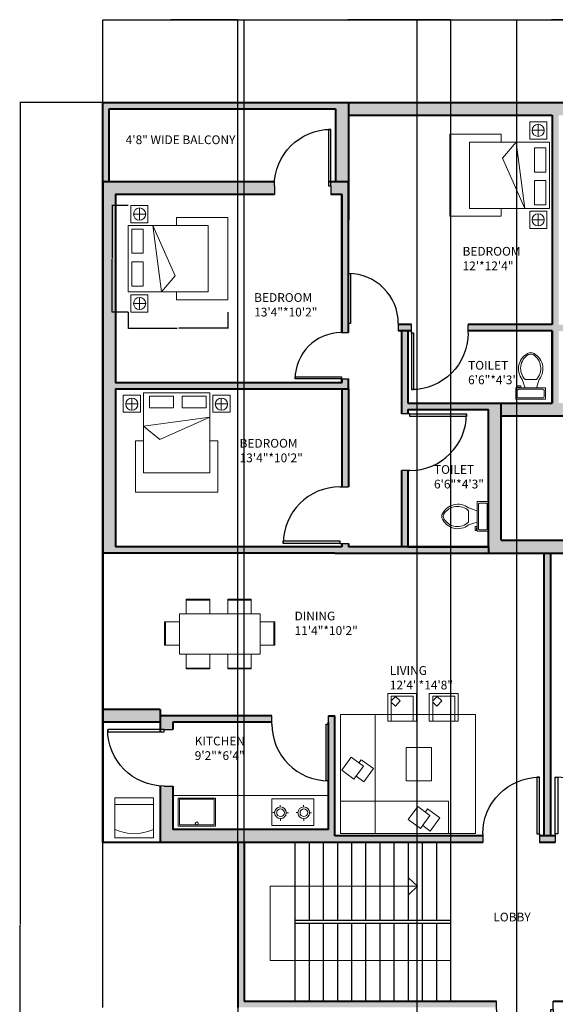
# Model space of a CAD drawing. Units: inches. Extents: x 1642 to 2399, y 1011 to 2291.
# Tile 4 of 7: x 1642 to 2020, y 1595 to 2291. Entities that reach past the tile are written whole.
import ezdxf

# ---------------------------------------------------------------- set-up
doc = ezdxf.new("R2010")
doc.units = ezdxf.units.IN
for name, color, linetype, lineweight in [('A-ANNO-DIMS', 2, 'Continuous', 18), ('A-ANNO-SYMB', 2, 'Continuous', 18), ('A-AREA-IDEN', 7, 'Continuous', 20), ('A-DOOR', 4, 'Continuous', 25), ('A-EQPM', 8, 'Continuous', 18), ('A-FLOR-CASE', 30, 'Continuous', 18), ('A-FLOR-FIXT', 9, 'Continuous', 18), ('A-FLOR-STRS', 7, 'Continuous', 25), ('A-FURN', 8, 'Continuous', 18), ('A-WALL-PATT', 40, 'Continuous', 13), ('BED', 200, 'Continuous', 18), ('WALL', 40, 'Continuous', 40)]:
    doc.layers.add(name, color=color, linetype=linetype, lineweight=lineweight)
doc.styles.get("Standard").update_dxf_attribs({"font": 'arial.ttf'})
doc.dimstyles.get("Standard").update_dxf_attribs({"dimtxt": 0.18, "dimasz": 0.18, "dimexe": 0.18, "dimexo": 0.0625, "dimgap": 0.09, "dimtad": 0, "dimtih": 1, "dimtoh": 1, "dimdec": 4, "dimzin": 0, "dimdsep": 46, "dimtxsty": 'Standard', "dimcen": 0.09, "dimadec": 0, "dimazin": 0, "dimtfac": 1, "dimtdec": 4, "dimtofl": 0, "dimtmove": 0, "dimatfit": 3, "dimfxl": 1, "dimtolj": 1, "dimtzin": 0, "dimarcsym": 0})

# ---------------------------------------------------------------- blocks, each defined once
blk = doc.blocks.new('*U2')
for p, q in [((0, 0), (0, -6)), ((40, 0), (40, -6))]:
    blk.add_line(p, q)
blk.add_lwpolyline([(0, 0), (0, 40), (1.75, 40), (1.75, 0)], close=True)
blk.add_arc((0, 0), 40, 0, 90)
blk = doc.blocks.new('*U4')
for p, q in [((9.5, -6), (9.5, -2)), ((-10, -8.5), (-8, -8.5)), ((-10, -9.5), (-10, -8.5)), ((-7, -9.5), (-10, -9.5)), ((-8, -8.5), (-8, -8)), ((-7, -8), (-7, -9.5)), ((-4, -8), (-6, -14)), ((4, -8), (6, -14)), ((4, -14), (-4, -14))]:
    blk.add_line(p, q)
blk.add_lwpolyline([(10.5, -8), (10.5, 0), (-10.5, 0), (-10.5, -8)], close=True)
for points in [[(-9.5, -2), (-9.5, -6)], [(8.5, -1), (-8.5, -1)], [(-8.5, -7), (8.5, -7)]]:
    blk.add_lwpolyline(points)
for centre, radius, start, end in [((-8.62, -1.88), 0.884, 81.8699, 188.1301), ((-8.62, -6.12), 0.884, 171.8699, 278.1301), ((8.62, -1.88), 0.884, 351.8699, 98.1301), ((8.62, -6.12), 0.884, 261.8699, 8.1301), ((3.52, -21.58), 12.17, 141.46911, 247.97143), ((4.2, -21.82), 11.33, 136.36773, 238.94682), ((-3.52, -21.58), 12.17, 292.02843, 38.53071), ((-4.2, -21.82), 11.33, 301.05301, 43.63209), ((0, -27.88), 4, 245.73182, 294.26817), ((0, -29), 4, 254.86053, 285.13947)]:
    blk.add_arc(centre, radius, start, end)
blk = doc.blocks.new('BED-DOUBLE-WITH-NIGHTSTANDS')
for p, q in [((8.62, 34.13), (8.62, 70.38)), ((8.62, 70.38), (66.79, 70.38)), ((66.79, 70.38), (66.79, 34.13)), ((14.22, 34.13), (8.62, 34.13)), ((14.22, 17.36), (49.69, 33.17)), ((49.69, 33.17), (61.11, 23.59)), ((66.79, 34.13), (61.11, 34.13)), ((61.11, 23.59), (14.22, 17.36)), ((1.82, 7.94), (10.42, 7.94)), ((6.17, 3.76), (6.17, 12.35)), ((65.06, 7.94), (73.65, 7.94)), ((69.41, 3.76), (69.41, 12.35))]:
    blk.add_line(p, q)
for points in [[(14.22, 0), (61.11, 0), (61.11, 56.52), (14.22, 56.52)], [(12.24, 1.79), (0, 1.79), (0, 13.82), (12.24, 13.82)], [(16.77, 2.51), (33.87, 2.51), (33.87, 10.66), (16.77, 10.66)], [(39.94, 2.51), (57.04, 2.51), (57.04, 10.66), (39.94, 10.66)], [(75.48, 1.79), (63.24, 1.79), (63.24, 13.82), (75.48, 13.82)]]:
    blk.add_lwpolyline(points, close=True)
for centre in [(6.12, 8.05), (69.36, 8.05)]:
    blk.add_circle(centre, 4.3)
blk = doc.blocks.new('TABLE-DINING-SIX-SEAT')
for p, q in [((15.31, 48.55), (31.81, 48.55)), ((44.68, 48.55), (61.18, 48.55)), ((0.59, 16.67), (0.59, 33.17)), ((77.22, 16.83), (77.22, 33.33)), ((15.31, 0.59), (31.81, 0.59)), ((44.68, 0.59), (61.18, 0.59))]:
    blk.add_line(p, q)
for points in [[(15.31, 38.77), (31.81, 38.77), (31.81, 49.15), (15.31, 49.15)], [(44.68, 38.77), (61.18, 38.77), (61.18, 49.15), (44.68, 49.15)], [(10.38, 38.77), (67.43, 38.77), (67.43, 10.38), (10.38, 10.38)], [(10.38, 16.67), (10.38, 33.17), (0, 33.17), (0, 16.67)], [(67.43, 16.83), (67.43, 33.33), (77.81, 33.33), (77.81, 16.83)], [(15.31, 10.38), (31.81, 10.38), (31.81, 0), (15.31, 0)], [(44.68, 10.38), (61.18, 10.38), (61.18, 0), (44.68, 0)]]:
    blk.add_lwpolyline(points, close=True)
blk = doc.blocks.new('SEATING-CORNER')
for points in [[(0, 84.13), (76.26, 84.13), (76.26, 61.34), (0, 61.34)], [(0, 0), (24.56, 0), (24.56, 84.13), (0, 84.13)], [(56.51, 80.66), (63.26, 71.39), (54.61, 65.09), (47.86, 74.37)], [(9.57, 45.8), (16.32, 36.53), (7.67, 30.23), (0.92, 39.51)]]:
    blk.add_lwpolyline(points, close=True)
for points in [[(58.1, 78.48), (63.51, 82.42), (70.26, 73.15), (61.61, 66.85), (60.02, 69.03)], [(11.16, 43.62), (16.57, 47.56), (23.32, 38.28), (14.67, 31.99), (13.08, 34.17)]]:
    blk.add_lwpolyline(points)
blk = doc.blocks.new('CHAIR-LOUNGE')
for p, q in [((2.54, 19.51), (0, 19.51)), ((0, 19.51), (0, 0)), ((18.08, 19.51), (20.31, 19.51)), ((20.31, 19.32), (20.31, 19.51)), ((20.31, 0), (20.31, 19.32)), ((0, 0), (20.31, 0))]:
    blk.add_line(p, q)
blk.add_lwpolyline([(2.54, 19.51), (18.08, 19.51), (18.08, 1.93), (2.54, 1.93)], close=True)
blk.add_lwpolyline([(2.54, 6.05), (5.4, 8.82), (8.88, 5.23), (5.55, 2), (2.54, 5.1)])
blk = doc.blocks.new('COOKTOP-TWO-BURNER')
for p, q in [((6.17, 13.89), (6.17, 15.59)), ((22.64, 13.89), (22.64, 15.59)), ((2, 9.67), (0.69, 9.67)), ((10.24, 9.72), (11.69, 9.72)), ((18.47, 9.67), (17.17, 9.67)), ((26.71, 9.72), (28.17, 9.72)), ((6.02, 5.65), (6.02, 4.35)), ((22.49, 5.65), (22.49, 4.35))]:
    blk.add_line(p, q)
blk.add_lwpolyline([(0, 18.89), (29.66, 18.89), (29.66, 0), (0, 0)], close=True)
for centre, radius in [((6.12, 9.77), 4.12), ((6.17, 9.77), 2.71), ((22.59, 9.77), 4.12), ((22.64, 9.77), 2.71)]:
    blk.add_circle(centre, radius)
blk = doc.blocks.new('SINK-KITCHEN-SINGLE')
for points in [[(0, 19.82), (26.24, 19.82), (26.24, 0), (0, 0)], [(0.83, 18.98), (25.41, 18.98), (25.41, 0.83), (0.83, 0.83)]]:
    blk.add_lwpolyline(points, close=True)
blk.add_circle((13.12, 17.93), 1.05)
blk = doc.blocks.new('UTILITY-APPLIANCE')
blk.add_line((0, 4.7), (27.35, 4.7))
blk.add_lwpolyline([(0, 28.26), (27.35, 28.26), (27.35, 0), (0, 0)], close=True)
blk.add_arc((13.68, -6.28), 31.65, 64.3994, 115.6006)
blk = doc.blocks.new('TABLE-COFFEE')
blk.add_lwpolyline([(0, 23.65), (17.89, 23.65), (17.89, 0), (0, 0)], close=True)
blk = doc.blocks.new('*D14')
at = {"layer": 'A-ANNO-DIMS', "color": 0, "lineweight": -2, "transparency": 16777216}
for p, q in [((1718.62, 2159.7), (1707.18, 2159.7)), ((1707.36, 2159.52), (1707.36, 2122.14)), ((1707.36, 2084.4), (1707.36, 2121.78)), ((1718.62, 2084.22), (1707.18, 2084.22))]:
    blk.add_line(p, q, dxfattribs=at)
at = {"layer": 'A-ANNO-DIMS', "color": 0, "transparency": 16777216}
for points in [[(1707.33, 2159.52), (1707.39, 2159.52), (1707.36, 2159.7)], [(1707.33, 2084.4), (1707.39, 2084.4), (1707.36, 2084.22)]]:
    blk.add_solid(points, dxfattribs=at)
at = {"layer": 'Defpoints', "color": 0, "transparency": 16777216}
for p in [(1718.68, 2159.7), (1707.36, 2084.22), (1718.68, 2084.22)]:
    blk.add_point(p, dxfattribs=at)
at = {"layer": 'A-ANNO-DIMS', "color": 0, "transparency": 16777216, "insert": (1707.36, 2121.96), "char_height": 0.18, "attachment_point": 5}
blk.add_mtext('\\A1;BED 75 TYP.', dxfattribs=at)
blk = doc.blocks.new('*D15')
at = {"layer": 'A-ANNO-DIMS', "color": 0, "lineweight": -2, "transparency": 16777216}
for p, q in [((1718.68, 2084.16), (1718.68, 2072.72)), ((1789.06, 2084.16), (1789.06, 2072.72)), ((1718.86, 2072.9), (1753.35, 2072.9)), ((1788.88, 2072.9), (1754.4, 2072.9))]:
    blk.add_line(p, q, dxfattribs=at)
at = {"layer": 'A-ANNO-DIMS', "color": 0, "transparency": 16777216}
for points in [[(1718.86, 2072.93), (1718.86, 2072.87), (1718.68, 2072.9)], [(1788.88, 2072.93), (1788.88, 2072.87), (1789.06, 2072.9)]]:
    blk.add_solid(points, dxfattribs=at)
at = {"layer": 'Defpoints', "color": 0, "transparency": 16777216}
for p in [(1718.68, 2084.22), (1789.06, 2084.22), (1789.06, 2072.9)]:
    blk.add_point(p, dxfattribs=at)
at = {"layer": 'A-ANNO-DIMS', "color": 0, "transparency": 16777216, "insert": (1753.87, 2072.9), "char_height": 0.18, "attachment_point": 5}
blk.add_mtext('\\A1;70 TYP.', dxfattribs=at)
blk = doc.blocks.new('*D32')
at = {"layer": 'A-ANNO-DIMS', "color": 0, "lineweight": -2, "transparency": 16777216}
for p, q in [((1700.71, 2232.52), (1700.71, 2290.98)), ((1700.89, 2290.8), (2020.07, 2290.8)), ((2340.03, 2290.8), (2020.86, 2290.8)), ((2340.21, 2232.52), (2340.21, 2290.98))]:
    blk.add_line(p, q, dxfattribs=at)
at = {"layer": 'A-ANNO-DIMS', "color": 0, "transparency": 16777216}
for points in [[(1700.89, 2290.83), (1700.89, 2290.77), (1700.71, 2290.8)], [(2340.03, 2290.83), (2340.03, 2290.77), (2340.21, 2290.8)]]:
    blk.add_solid(points, dxfattribs=at)
at = {"layer": 'Defpoints', "color": 0, "transparency": 16777216}
for p in [(2340.21, 2290.8), (1700.71, 2232.46), (2340.21, 2232.46)]:
    blk.add_point(p, dxfattribs=at)
at = {"layer": 'A-ANNO-DIMS', "color": 0, "transparency": 16777216, "insert": (2020.46, 2290.8), "char_height": 0.18, "attachment_point": 5}
blk.add_mtext('\\A1;639.5', dxfattribs=at)
blk = doc.blocks.new('*D33')
at = {"layer": 'A-ANNO-DIMS', "color": 0, "lineweight": -2, "transparency": 16777216}
for p, q in [((1700.65, 2232.46), (1642.19, 2232.46)), ((1642.37, 2232.28), (1642.37, 1651.26)), ((1642.37, 1069.89), (1642.37, 1650.9)), ((1700.65, 1069.71), (1642.19, 1069.71))]:
    blk.add_line(p, q, dxfattribs=at)
at = {"layer": 'A-ANNO-DIMS', "color": 0, "transparency": 16777216}
for points in [[(1642.34, 2232.28), (1642.4, 2232.28), (1642.37, 2232.46)], [(1642.34, 1069.89), (1642.4, 1069.89), (1642.37, 1069.71)]]:
    blk.add_solid(points, dxfattribs=at)
at = {"layer": 'Defpoints', "color": 0, "transparency": 16777216}
for p in [(1642.37, 2232.46), (1700.71, 2232.46), (1700.71, 1069.71)]:
    blk.add_point(p, dxfattribs=at)
at = {"layer": 'A-ANNO-DIMS', "color": 0, "transparency": 16777216, "insert": (1642.37, 1651.08), "char_height": 0.18, "attachment_point": 5}
blk.add_mtext('\\A1;1162.7', dxfattribs=at)
blk = doc.blocks.new('*D39')
at = {"layer": 'A-ANNO-DIMS', "color": 0, "lineweight": -2, "transparency": 16777216}
for p, q in [((1700.71, 1592.77), (1700.71, 2290.98)), ((1700.89, 2290.8), (1748.05, 2290.8)), ((1796, 2290.8), (1748.84, 2290.8)), ((1796.18, 1592.77), (1796.18, 2290.98))]:
    blk.add_line(p, q, dxfattribs=at)
at = {"layer": 'A-ANNO-DIMS', "color": 0, "transparency": 16777216}
for points in [[(1700.89, 2290.83), (1700.89, 2290.77), (1700.71, 2290.8)], [(1796, 2290.83), (1796, 2290.77), (1796.18, 2290.8)]]:
    blk.add_solid(points, dxfattribs=at)
at = {"layer": 'Defpoints', "color": 0, "transparency": 16777216}
for p in [(1796.18, 2290.8), (1700.71, 1592.71), (1796.18, 1592.71)]:
    blk.add_point(p, dxfattribs=at)
at = {"layer": 'A-ANNO-DIMS', "color": 0, "transparency": 16777216, "insert": (1748.45, 2290.8), "char_height": 0.18, "attachment_point": 5}
blk.add_mtext('\\A1;95.47', dxfattribs=at)
blk = doc.blocks.new('*D40')
at = {"layer": 'A-ANNO-DIMS', "color": 0, "lineweight": -2, "transparency": 16777216}
for p, q in [((1796.18, 1709.39), (1796.18, 1011.19)), ((2186.88, 1709.39), (2186.88, 1011.19)), ((1796.36, 1011.37), (1991.13, 1011.37)), ((2186.7, 1011.37), (1991.92, 1011.37))]:
    blk.add_line(p, q, dxfattribs=at)
at = {"layer": 'A-ANNO-DIMS', "color": 0, "transparency": 16777216}
for points in [[(1796.36, 1011.4), (1796.36, 1011.34), (1796.18, 1011.37)], [(2186.7, 1011.4), (2186.7, 1011.34), (2186.88, 1011.37)]]:
    blk.add_solid(points, dxfattribs=at)
at = {"layer": 'Defpoints', "color": 0, "transparency": 16777216}
for p in [(1796.18, 1709.46), (2186.88, 1709.46), (2186.88, 1011.37)]:
    blk.add_point(p, dxfattribs=at)
at = {"layer": 'A-ANNO-DIMS', "color": 0, "transparency": 16777216, "insert": (1991.53, 1011.37), "char_height": 0.18, "attachment_point": 5}
blk.add_mtext('\\A1;390.7', dxfattribs=at)
blk = doc.blocks.new('*D41')
at = {"layer": 'A-ANNO-DIMS', "color": 0, "lineweight": -2, "transparency": 16777216}
for p, q in [((1800.68, 1597.27), (1800.68, 2290.98)), ((1800.86, 2290.8), (1873.4, 2290.8)), ((1946.5, 2290.8), (1873.96, 2290.8)), ((1946.68, 1597.27), (1946.68, 2290.98))]:
    blk.add_line(p, q, dxfattribs=at)
at = {"layer": 'A-ANNO-DIMS', "color": 0, "transparency": 16777216}
for points in [[(1800.86, 2290.83), (1800.86, 2290.77), (1800.68, 2290.8)], [(1946.5, 2290.83), (1946.5, 2290.77), (1946.68, 2290.8)]]:
    blk.add_solid(points, dxfattribs=at)
at = {"layer": 'Defpoints', "color": 0, "transparency": 16777216}
for p in [(1946.68, 2290.8), (1800.68, 1597.21), (1946.68, 1597.21)]:
    blk.add_point(p, dxfattribs=at)
at = {"layer": 'A-ANNO-DIMS', "color": 0, "transparency": 16777216, "insert": (1873.68, 2290.8), "char_height": 0.18, "attachment_point": 5}
blk.add_mtext('\\A1;146', dxfattribs=at)
blk = doc.blocks.new('*D42')
at = {"layer": 'A-ANNO-DIMS', "color": 0, "lineweight": -2, "transparency": 16777216}
for p, q in [((1946.68, 1597.27), (1946.68, 2290.98)), ((1946.86, 2290.8), (2016.99, 2290.8)), ((2087.89, 2290.8), (2017.76, 2290.8)), ((2088.07, 1597.27), (2088.07, 2290.98))]:
    blk.add_line(p, q, dxfattribs=at)
at = {"layer": 'A-ANNO-DIMS', "color": 0, "transparency": 16777216}
for points in [[(1946.86, 2290.83), (1946.86, 2290.77), (1946.68, 2290.8)], [(2087.89, 2290.83), (2087.89, 2290.77), (2088.07, 2290.8)]]:
    blk.add_solid(points, dxfattribs=at)
at = {"layer": 'Defpoints', "color": 0, "transparency": 16777216}
for p in [(2088.07, 2290.8), (1946.68, 1597.21), (2088.07, 1597.21)]:
    blk.add_point(p, dxfattribs=at)
at = {"layer": 'A-ANNO-DIMS', "color": 0, "transparency": 16777216, "insert": (2017.37, 2290.8), "char_height": 0.18, "attachment_point": 5}
blk.add_mtext('\\A1;141.4', dxfattribs=at)
blk = doc.blocks.new('*D48')
at = {"layer": 'A-ANNO-DIMS', "color": 0, "lineweight": -2, "transparency": 16777216}
for p, q in [((1922.74, 1392.77), (1922.74, 2290.98)), ((1922.92, 2290.8), (2031.1, 2290.8)), ((2140.06, 2290.8), (2031.89, 2290.8)), ((2140.24, 1392.77), (2140.24, 2290.98))]:
    blk.add_line(p, q, dxfattribs=at)
at = {"layer": 'A-ANNO-DIMS', "color": 0, "transparency": 16777216}
for points in [[(1922.92, 2290.83), (1922.92, 2290.77), (1922.74, 2290.8)], [(2140.06, 2290.83), (2140.06, 2290.77), (2140.24, 2290.8)]]:
    blk.add_solid(points, dxfattribs=at)
at = {"layer": 'Defpoints', "color": 0, "transparency": 16777216}
for p in [(2140.24, 2290.8), (1922.74, 1392.71), (2140.24, 1392.71)]:
    blk.add_point(p, dxfattribs=at)
at = {"layer": 'A-ANNO-DIMS', "color": 0, "transparency": 16777216, "insert": (2031.49, 2290.8), "char_height": 0.18, "attachment_point": 5}
blk.add_mtext('\\A1;217.5', dxfattribs=at)
blk = doc.blocks.new('*D50')
at = {"layer": 'A-ANNO-DIMS', "color": 0, "lineweight": -2, "transparency": 16777216}
for p, q in [((1993.24, 1295.77), (1993.24, 2290.98)), ((1993.42, 2290.8), (2031.17, 2290.8)), ((2069.56, 2290.8), (2031.82, 2290.8)), ((2069.74, 1295.77), (2069.74, 2290.98))]:
    blk.add_line(p, q, dxfattribs=at)
at = {"layer": 'A-ANNO-DIMS', "color": 0, "transparency": 16777216}
for points in [[(1993.42, 2290.83), (1993.42, 2290.77), (1993.24, 2290.8)], [(2069.56, 2290.83), (2069.56, 2290.77), (2069.74, 2290.8)]]:
    blk.add_solid(points, dxfattribs=at)
at = {"layer": 'Defpoints', "color": 0, "transparency": 16777216}
for p in [(2069.74, 2290.8), (1993.24, 1295.71), (2069.74, 1295.71)]:
    blk.add_point(p, dxfattribs=at)
at = {"layer": 'A-ANNO-DIMS', "color": 0, "transparency": 16777216, "insert": (2031.49, 2290.8), "char_height": 0.18, "attachment_point": 5}
blk.add_mtext('\\A1;76.5', dxfattribs=at)

msp = doc.modelspace()

# ---------------------------------------------------------------- hatches: boundary and pattern name
at = {"layer": 'A-WALL-PATT'}
h = msp.add_hatch(color=256, dxfattribs=at)
h.dxf.hatch_style = 1
h.paths.add_polyline_path([(2340.1804, 2185.4562), (2211.0983, 2185.4562, -0.01876983), (2211.211, 2182.4562), (2211.211, 2176.4562), (2331.211, 2176.4562), (2331.211, 2043.4562), (2171.211, 2043.4562), (2171.211, 2038.9562), (2331.211, 2038.9562), (2331.211, 1916.9562), (2171.211, 1916.9562), (2171.211, 1918.9365), (2166.711, 1918.9365), (2166.711, 1912.4562), (2340.1804, 1912.4562)])
h.paths.add_polyline_path([(2171.211, 2043.4562), (2171.211, 2043.9025), (2170.5217, 2043.9025), (2166.711, 2043.9025), (2166.711, 2038.9562), (2166.711, 1958.9365), (2171.211, 1958.9365)], flags=17)
h.paths.add_polyline_path([(2129.211, 1971.5979), (2124.711, 1971.5979), (2124.711, 1918.4562), (2067.711, 1918.4562), (2067.711, 1913.9562), (2129.211, 1913.9562)])
h.paths.add_polyline_path([(2067.711, 2015.4562), (2124.711, 2015.4562), (2124.711, 2019.9562), (2058.711, 2019.9562), (2058.711, 2015.4562), (2058.711, 1922.9562), (1982.211, 1922.9562), (1982.211, 2015.4562), (1982.211, 2019.9562), (1916.211, 2019.9562), (1916.211, 2070.9562), (1911.711, 2070.9562), (1911.711, 2015.4562), (1911.711, 2012.302), (1916.211, 2012.302), (1916.211, 2015.4562), (1973.211, 2015.4562), (1973.211, 1918.4562), (1973.211, 1913.9562), (2017.1804, 1913.9562), (2067.711, 1913.9562), (2067.711, 1918.4562)])
h.paths.add_polyline_path([(2131.1386, 2075.4562), (2118.1934, 2075.4562), (2118.1934, 2070.9562), (2131.1386, 2070.9562)], flags=17)
h.paths.add_polyline_path([(1918.8034, 2075.4562), (1909.4956, 2075.4562), (1909.4956, 2070.9562), (1918.8034, 2070.9562)], flags=17)
h.paths.add_polyline_path([(1874.211, 2029.9562), (1869.711, 2029.9562), (1869.711, 1960.7404), (1874.211, 1960.7404)], flags=17)
h.paths.add_polyline_path([(1916.211, 1972.302), (1911.711, 1972.302), (1911.711, 1918.4562), (1916.211, 1918.4562)], flags=17)
h.paths.add_polyline_path([(2340.1804, 1912.4562), (2331.1804, 1912.4562), (2331.1804, 1794.4562), (2210.1804, 1794.4562), (2210.1804, 1789.9562), (2279.6804, 1789.9562), (2340.1804, 1789.9562)])
h.paths.add_polyline_path([(2288.6804, 1789.9562), (2279.6804, 1789.9562), (2279.6804, 1785.0846), (2285.6804, 1785.0846), (2288.6804, 1785.0846)], flags=17)
h.paths.add_polyline_path([(2169.6804, 1789.9562), (2170.1804, 1789.9562), (2170.1804, 1794.4562), (2165.1804, 1794.4562), (2165.1804, 1713.9562), (2165.1804, 1709.4562), (2279.6804, 1709.4562), (2279.6804, 1718.4562), (2169.6804, 1718.4562)])
h.paths.add_polyline_path([(2288.6804, 1745.1973, -0.01876983), (2285.6804, 1745.0846), (2279.6804, 1745.0846), (2279.6804, 1709.4562), (2340.1804, 1709.4562), (2340.1804, 1789.9562), (2335.6804, 1789.9562), (2335.6804, 1713.9562), (2288.6804, 1713.9562)])
h.paths.add_polyline_path([(2165.1804, 1713.9562), (2140.6229, 1713.9562), (2088.923, 1713.9562), (2069.7509, 1713.9562), (2060.4457, 1713.9562), (2060.4457, 1709.4562), (2165.1804, 1709.4562)])
h.paths.add_polyline_path([(2020.4457, 1713.9562), (2017.1804, 1713.9562), (2012.6804, 1713.9562), (2009.1946, 1713.9562), (2009.1946, 1709.4562), (2020.4457, 1709.4562)])
h.paths.add_polyline_path([(1969.1946, 1713.9562), (1864.6804, 1713.9562), (1864.6804, 1798.9562), (1860.1804, 1798.9562), (1860.1804, 1792.9562), (1860.1804, 1752.9562), (1860.1804, 1718.4562), (1750.1804, 1718.4562), (1750.1804, 1749.2419), (1744.1804, 1749.2419, -0.01876983), (1741.1804, 1749.3546), (1741.1804, 1709.4562), (1969.1946, 1709.4562)])
h.paths.add_polyline_path([(1741.1804, 1803.4562), (1700.711, 1803.4562), (1700.711, 1794.4562), (1741.1804, 1794.4562)])
h.paths.add_polyline_path([(1820.1804, 1798.9562), (1741.1804, 1798.9562), (1741.1804, 1794.4562), (1741.1804, 1790.0365), (1741.1804, 1789.2419), (1744.1804, 1789.2419), (1750.1804, 1789.2419), (1750.1804, 1794.4562), (1820.1804, 1794.4562)], flags=17)
h.paths.add_polyline_path([(1800.6804, 1709.4562), (1796.1804, 1709.4562), (1796.1804, 1592.7078), (1978.9325, 1592.7078), (1978.9325, 1597.2078), (1800.6804, 1597.2078)])
h.paths.add_polyline_path([(2097.0678, 1709.4562), (2088.0678, 1709.4562), (2088.0678, 1599.6874), (2088.0678, 1597.2078), (2097.0678, 1597.2078)], flags=17)
h.paths.add_polyline_path([(2186.8766, 1709.4562), (2182.3766, 1709.4562), (2182.3766, 1597.2078), (2071.4624, 1597.2078), (2071.4624, 1592.7078), (2186.8766, 1592.7078)])
h.paths.add_polyline_path([(2078.1934, 2075.4562), (2022.711, 2075.4562), (2022.711, 2223.4562), (2166.711, 2223.4562), (2166.711, 2075.4562), (2166.711, 2070.9562), (2171.211, 2070.9562), (2171.211, 2138.8919), (2171.211, 2227.9562), (2335.711, 2227.9562), (2335.711, 2185.4562), (2340.1804, 2185.4562), (2340.1804, 2232.4562), (1874.211, 2232.4562), (1874.211, 2223.4562), (2018.211, 2223.4562), (2018.211, 2075.4562), (1958.8034, 2075.4562), (1958.8034, 2070.9562), (2018.211, 2070.9562), (2018.211, 2019.9562), (1982.211, 2019.9562), (1982.211, 2015.4562), (1982.211, 2010.9562), (2058.711, 2010.9562), (2058.711, 2015.4562), (2058.711, 2019.9562), (2022.711, 2019.9562), (2022.711, 2070.9562), (2078.1934, 2070.9562)])
h.paths.add_polyline_path([(1874.211, 2171.9562), (1874.211, 2176.4562), (1861.9371, 2176.4562), (1861.9371, 2173.4562), (1861.9371, 2167.4562), (1869.711, 2167.4562), (1869.711, 2069.7602), (1874.211, 2069.7602)], flags=17)
h.paths.add_polyline_path([(1705.211, 2227.9562), (1865.211, 2227.9562), (1865.211, 2176.4562), (1874.211, 2176.4562), (1874.211, 2232.4562), (1700.711, 2232.4562), (1700.711, 2176.4562), (1705.211, 2176.4562)])
h.paths.add_polyline_path([(1709.711, 2167.4562), (1821.9371, 2167.4562), (1821.9371, 2173.4562, -0.01876983), (1822.0498, 2176.4562), (1700.711, 2176.4562), (1700.711, 1913.9562), (1860.1804, 1913.9562), (1864.6804, 1913.9562), (1973.211, 1913.9562), (1973.211, 1918.4562), (1916.211, 1918.4562), (1874.211, 1918.4562), (1874.211, 1920.7404), (1869.711, 1920.7404), (1869.711, 1918.4562), (1860.1804, 1918.4562), (1709.711, 1918.4562), (1709.711, 2029.9562), (1874.211, 2029.9562), (1874.211, 2037.0364), (1869.711, 2037.0364), (1869.711, 2034.4562), (1709.711, 2034.4562)])
h.paths.add_polyline_path([(2017.1804, 1913.9562), (2012.6804, 1913.9562), (2012.6804, 1713.9562), (2017.1804, 1713.9562)])
h.paths.add_polyline_path([(1952.4341, 2110.3716), (2000.4134, 2110.3716), (2000.4134, 2133.4189), (1952.4341, 2133.4189)], flags=25)
h.paths.add_polyline_path([(2042.3983, 2110.7121), (2090.3775, 2110.7121), (2090.3775, 2133.7594), (2042.3983, 2133.7594)], flags=25)
h.paths.add_polyline_path([(2201.7332, 2091.8715), (2249.7125, 2091.8715), (2249.7125, 2114.9188), (2201.7332, 2114.9188)], flags=25)
h.paths.add_polyline_path([(1805.186, 2077.6915), (1853.1653, 2077.6915), (1853.1653, 2100.7388), (1805.186, 2100.7388)], flags=25)
h.paths.add_polyline_path([(1794.8897, 1974.6584), (1842.869, 1974.6584), (1842.869, 1997.7057), (1794.8897, 1997.7057)], flags=25)
h.paths.add_polyline_path([(2229.1796, 2204.4209), (2315.1362, 2204.4209), (2315.1362, 2217.1488), (2229.1796, 2217.1488)], flags=25)
h.paths.add_polyline_path([(1715.2159, 2199.5328), (1801.1724, 2199.5328), (1801.1724, 2212.2607), (1715.2159, 2212.2607)], flags=25)
h.paths.add_polyline_path([(2230.7681, 1755.7109), (2271.7283, 1755.7109), (2271.7283, 1778.7582), (2230.7681, 1778.7582)], flags=25)
h.paths.add_polyline_path([(1763.4713, 1764.1742), (1804.4315, 1764.1742), (1804.4315, 1787.2215), (1763.4713, 1787.2215)], flags=25)
h.paths.add_polyline_path([(2076.2643, 1955.0495), (2111.326, 1955.0495), (2111.326, 1978.0968), (2076.2643, 1978.0968)], flags=25)
h.paths.add_polyline_path([(1932.854, 1956.1217), (1967.9158, 1956.1217), (1967.9158, 1979.169), (1932.854, 1979.169)], flags=25)
h.paths.add_polyline_path([(2048.1203, 2031.6107), (2083.1821, 2031.6107), (2083.1821, 2054.658), (2048.1203, 2054.658)], flags=25)
h.paths.add_polyline_path([(2163.5754, 1863.7569), (2208.2347, 1863.7569), (2208.2347, 1886.8042), (2163.5754, 1886.8042)], flags=9)
h.paths.add_polyline_path([(2039.9286, 1809.0957), (2084.5879, 1809.0957), (2084.5879, 1832.143), (2039.9286, 1832.143)], flags=9)
h.paths.add_polyline_path([(1901.0045, 1814.0452), (1945.6638, 1814.0452), (1945.6638, 1837.0925), (1901.0045, 1837.0925)], flags=9)
h.paths.add_polyline_path([(1833.7282, 1852.5627), (1878.3875, 1852.5627), (1878.3875, 1875.61), (1833.7282, 1875.61)], flags=9)
h.paths.add_polyline_path([(2219.1375, 1926.2139), (2267.1167, 1926.2139), (2267.1167, 1949.2612), (2219.1375, 1949.2612)], flags=25)
h.paths.add_polyline_path([(1956.9598, 2029.7735), (1992.0216, 2029.7735), (1992.0216, 2052.8208), (1956.9598, 2052.8208)], flags=25)
h.paths.add_polyline_path([(2229.3, 1523.3399), (2270.2602, 1523.3399), (2270.2602, 1546.3872), (2229.3, 1546.3872)], flags=9)
h.paths.add_polyline_path([(1772.3039, 1526.9922), (1813.2641, 1526.9922), (1813.2641, 1550.0394), (1772.3039, 1550.0394)], flags=9)
h.paths.add_polyline_path([(2172.587, 1420.6999), (2217.2463, 1420.6999), (2217.2463, 1443.7472), (2172.587, 1443.7472)], flags=9)
h.paths.add_polyline_path([(1814.3549, 1422.215), (1859.0143, 1422.215), (1859.0143, 1445.2623), (1814.3549, 1445.2623)], flags=9)
h.paths.add_polyline_path([(2186.0372, 1305.6227), (2234.0165, 1305.6227), (2234.0165, 1328.67), (2186.0372, 1328.67)], flags=9)
h.paths.add_polyline_path([(1756.747, 1349.0694), (1804.7263, 1349.0694), (1804.7263, 1372.1167), (1756.747, 1372.1167)], flags=9)
h.paths.add_polyline_path([(2239.449, 1214.6184), (2287.4282, 1214.6184), (2287.4282, 1237.6657), (2239.449, 1237.6657)], flags=9)
h.paths.add_polyline_path([(1767.104, 1213.8348), (1815.0832, 1213.8348), (1815.0832, 1236.8821), (1767.104, 1236.8821)], flags=9)
h.paths.add_polyline_path([(2046.6809, 1183.6854), (2094.6602, 1183.6854), (2094.6602, 1206.7327), (2046.6809, 1206.7327)], flags=9)
h.paths.add_polyline_path([(1947.2155, 1183.6854), (1995.1948, 1183.6854), (1995.1948, 1206.7327), (1947.2155, 1206.7327)], flags=9)
h.paths.add_polyline_path([(1959.3556, 1258.7871), (1994.4174, 1258.7871), (1994.4174, 1281.8344), (1959.3556, 1281.8344)], flags=9)
h.paths.add_polyline_path([(2049.6419, 1248.9629), (2084.7036, 1248.9629), (2084.7036, 1272.0102), (2049.6419, 1272.0102)], flags=9)
h.paths.add_polyline_path([(2092.7532, 1327.4852), (2127.815, 1327.4852), (2127.815, 1350.5325), (2092.7532, 1350.5325)], flags=9)
h.paths.add_polyline_path([(1944.9358, 1327.4852), (1979.9976, 1327.4852), (1979.9976, 1350.5325), (1944.9358, 1350.5325)], flags=9)
h.paths.add_polyline_path([(1974.5055, 1650.063), (2006.3695, 1650.063), (2006.3695, 1662.7909), (1974.5055, 1662.7909)], flags=9)

# ---------------------------------------------------------------- linework, layer by layer
at = {"layer": 'A-ANNO-SYMB'}
for p, q in [((1923.0619, 1678.382), (1916.6804, 1684.4209)), ((1818.9958, 1626.0366), (1818.9958, 1678.382)), ((1818.9958, 1678.382), (1923.0619, 1678.382)), ((1923.0619, 1678.382), (1916.6804, 1672.3431)), ((1946.6804, 1626.0366), (1818.9958, 1626.0366))]:
    msp.add_line(p, q, dxfattribs=at)
at = {"layer": 'A-FLOR-CASE'}
msp.add_line((1750.1804, 1742.5391), (1860.1804, 1742.5391), dxfattribs=at)
at = {"layer": 'A-FLOR-STRS'}
for p, q in [((1836.6804, 1597.2078), (1836.6804, 1709.4562)), ((1846.6804, 1654.332), (1846.6804, 1709.4562)), ((1856.6804, 1654.332), (1856.6804, 1709.4562)), ((1866.6804, 1654.332), (1866.6804, 1709.4562)), ((1876.6804, 1654.332), (1876.6804, 1709.4562)), ((1886.6804, 1654.332), (1886.6804, 1709.4562)), ((1896.6804, 1654.332), (1896.6804, 1709.4562)), ((1906.6804, 1654.332), (1906.6804, 1709.4562)), ((1916.6804, 1654.332), (1916.6804, 1709.4562)), ((1926.6804, 1654.332), (1926.6804, 1709.4562)), ((1936.6804, 1654.332), (1936.6804, 1709.4562)), ((1946.6804, 1597.2078), (1946.6804, 1709.4562)), ((1836.6804, 1654.332), (1946.6804, 1654.332)), ((1836.6804, 1652.332), (1946.6804, 1652.332)), ((1846.6804, 1597.2078), (1846.6804, 1652.332)), ((1856.6804, 1597.2078), (1856.6804, 1652.332)), ((1866.6804, 1597.2078), (1866.6804, 1652.332)), ((1876.6804, 1597.2078), (1876.6804, 1652.332)), ((1886.6804, 1597.2078), (1886.6804, 1652.332)), ((1896.6804, 1597.2078), (1896.6804, 1652.332)), ((1906.6804, 1597.2078), (1906.6804, 1652.332)), ((1916.6804, 1597.2078), (1916.6804, 1652.332)), ((1926.6804, 1597.2078), (1926.6804, 1652.332)), ((1936.6804, 1597.2078), (1936.6804, 1652.332)), ((1800.6804, 1597.2078), (1836.6804, 1597.2078))]:
    msp.add_line(p, q, dxfattribs=at)
at = {"layer": 'A-FURN'}
msp.add_lwpolyline([(1868.6347, 1715.7451), (1964.0642, 1715.7451), (1964.0642, 1799.8733), (1868.6347, 1799.8733)], close=True, dxfattribs=at)
at = {"layer": 'WALL'}
for p, q in [((1700.711, 2176.4562), (1700.711, 2232.4562)), ((1700.711, 2232.4562), (1874.211, 2232.4562)), ((1705.211, 2176.4562), (1705.211, 2227.9562)), ((1705.211, 2227.9562), (1865.211, 2227.9562)), ((1865.211, 2227.9562), (1865.211, 2176.4562)), ((1874.211, 2232.4562), (1874.211, 2149.2118)), ((1874.211, 2232.4562), (2022.711, 2232.4562)), ((1874.211, 2223.4562), (2018.211, 2223.4562)), ((2018.211, 2223.4562), (2018.211, 2075.4562)), ((1869.711, 2167.4562), (1869.711, 2069.7602)), ((1918.8034, 2075.4562), (1909.4956, 2075.4562)), ((2018.211, 2075.4562), (1958.8034, 2075.4562)), ((1918.8034, 2070.9562), (1909.4956, 2070.9562)), ((1911.711, 2070.9562), (1911.711, 2015.4562)), ((1916.211, 2070.9562), (1916.211, 2019.9562)), ((2018.211, 2070.9562), (1958.8034, 2070.9562)), ((2018.211, 2070.9562), (2018.211, 2019.9562)), ((2018.211, 2019.9562), (2018.211, 2070.9562)), ((1869.711, 2037.0364), (1869.711, 2034.4562)), ((1700.711, 2029.9562), (1700.711, 1709.4562)), ((1709.711, 2029.9562), (1709.711, 1918.4562)), ((1869.711, 2029.9562), (1869.711, 1960.7404)), ((1874.211, 2029.9562), (1874.211, 1960.7404)), ((1916.211, 2019.9562), (2018.211, 2019.9562)), ((1982.211, 2015.4562), (1982.211, 2019.9562)), ((1911.711, 2015.4562), (1911.711, 2012.302)), ((1916.211, 2015.4562), (1973.211, 2015.4562)), ((1916.211, 2015.4562), (1916.211, 2012.302)), ((1973.211, 1918.4562), (1973.211, 2015.4562)), ((1982.211, 1922.9562), (1982.211, 2015.4562)), ((1982.211, 2010.9562), (2058.711, 2010.9562)), ((1911.711, 1972.302), (1911.711, 1918.4562)), ((1916.211, 1972.302), (1916.211, 1918.4562)), ((1982.211, 1922.9562), (2058.711, 1922.9562)), ((1860.1804, 1918.4562), (1709.711, 1918.4562)), ((1869.711, 1918.4562), (1860.1804, 1918.4562)), ((1869.711, 1920.7404), (1869.711, 1918.4562)), ((1874.211, 1920.7404), (1874.211, 1918.4562)), ((1973.211, 1918.4562), (1874.211, 1918.4562)), ((1916.211, 1918.4562), (1973.211, 1918.4562)), ((1973.211, 1918.4562), (1973.211, 1913.9562)), ((1860.1804, 1913.9562), (1700.711, 1913.9562)), ((1864.6804, 1913.9562), (1849.3611, 1913.9562)), ((1864.6804, 1913.9562), (2017.1804, 1913.9562)), ((2012.6804, 1713.9562), (2012.6804, 1913.9562)), ((2012.6804, 1913.9562), (2129.211, 1913.9562)), ((2017.1804, 1713.9562), (2017.1804, 1913.9562)), ((1741.1804, 1803.4562), (1700.711, 1803.4562)), ((1741.1804, 1803.4562), (1741.1804, 1790.0365)), ((1820.1804, 1798.9562), (1741.1804, 1798.9562)), ((1741.1804, 1798.9562), (1741.1804, 1787.4919)), ((1860.1804, 1798.9562), (1864.6804, 1798.9562)), ((1864.6804, 1713.9562), (1864.6804, 1798.9562)), ((1741.1804, 1794.4562), (1700.711, 1794.4562)), ((1820.1804, 1794.4562), (1750.1804, 1794.4562)), ((1750.1804, 1794.4562), (1750.1804, 1789.2419)), ((1860.1804, 1718.4562), (1860.1804, 1794.4562)), ((1860.1804, 1718.4562), (1860.1804, 1794.4562)), ((1741.1804, 1749.3546), (1741.1804, 1709.4562)), ((1750.1804, 1749.2419), (1750.1804, 1718.4562)), ((1860.1804, 1718.4562), (1750.1804, 1718.4562)), ((1969.1946, 1713.9562), (1864.6804, 1713.9562)), ((2012.6804, 1713.9562), (2009.1946, 1713.9562)), ((2020.4457, 1713.9562), (2012.6804, 1713.9562)), ((2020.4457, 1713.9562), (2017.1804, 1713.9562)), ((1741.1804, 1709.4562), (1700.711, 1709.4562)), ((1860.1804, 1709.4562), (1741.1804, 1709.4562)), ((1796.1804, 1709.4562), (1796.1804, 1592.7078)), ((1800.6804, 1709.4562), (1800.6804, 1597.2078)), ((1969.1946, 1709.4562), (1860.1804, 1709.4562)), ((2020.4457, 1709.4562), (2009.1946, 1709.4562)), ((1800.6804, 1597.2078), (1978.9325, 1597.2078)), ((2018.9325, 1597.2078), (2031.4624, 1597.2078))]:
    msp.add_line(p, q, dxfattribs=at)
for points in [[(1969.1946, 1709.4562), (1700.711, 1709.4562), (1700.711, 2232.4562), (2340.1804, 2232.4562), (2340.1804, 1709.4562), (2060.4457, 1709.4562)], [(1822.0498, 2176.4562), (1700.711, 2176.4562), (1700.711, 2029.9562)], [(1874.211, 2069.7602), (1874.211, 2176.4562), (1860.1871, 2176.4562)], [(1874.211, 2069.7602), (1874.211, 2171.9562)], [(1821.9371, 2167.4562), (1709.711, 2167.4562), (1709.711, 2034.4562), (1869.711, 2034.4562), (1869.711, 2037.0364)], [(1869.711, 2069.7602), (1869.711, 2167.4562), (1861.9371, 2167.4562)], [(1709.711, 2029.9562), (1874.211, 2029.9562), (1874.211, 2037.0364)], [(1874.211, 2034.4562), (1874.211, 2037.0364)], [(2020.4457, 1709.4562), (2009.1946, 1709.4562)]]:
    msp.add_lwpolyline(points, dxfattribs=at)

# ---------------------------------------------------------------- block references
at = {"layer": 'A-DOOR', "xscale": -1}
for p in [(1861.9371, 2173.4562), (2009.1946, 1715.4562)]:
    msp.add_blockref('*U2', p, dxfattribs=at)
at = {"layer": 'A-DOOR', "xscale": 0.8821151555057145, "yscale": 0.8821151555057145, "zscale": 0.8821151555057145}
msp.add_blockref('*U2', (1874.211, 2076.2489), dxfattribs=at)
at = {"layer": 'A-DOOR', "xscale": -1}
for p, rotation in [((1918.8034, 2069.4562), 180), ((1744.1804, 1789.2419), 90)]:
    msp.add_blockref('*U2', p, dxfattribs=dict(at, rotation=rotation))
at = {"layer": 'A-DOOR', "xscale": 0.8180946750226169, "yscale": 0.8180946750226169, "zscale": 0.8180946750226169, "rotation": 90}
msp.add_blockref('*U2', (1869.3024, 2037.0364), dxfattribs=at)
at = {"layer": 'A-DOOR'}
for p, rotation in [((1917.711, 2012.302), 270), ((1868.211, 1920.7404), 90), ((1860.1804, 1792.9562), 180), ((2018.9325, 1591.2078), 180)]:
    msp.add_blockref('*U2', p, dxfattribs=dict(at, rotation=rotation))
msp.add_blockref('*U2', (2020.4457, 1715.4562), dxfattribs=at)
at = {"layer": 'A-EQPM', "rotation": 180}
msp.add_blockref('UTILITY-APPLIANCE', (1736.4661, 1740.8892), dxfattribs=at)
at = {"layer": 'A-EQPM', "extrusion": (0, 0, -1), "zscale": -1, "rotation": 180}
msp.add_blockref('COOKTOP-TWO-BURNER', (-1820.1264, 1740.14), dxfattribs=at)
at = {"layer": 'A-FLOR-FIXT', "xscale": -1}
for p, rotation in [((2003.0765, 2022.682), 180), ((1973.211, 1939.8242), 270)]:
    msp.add_blockref('*U4', p, dxfattribs=dict(at, rotation=rotation))
at = {"layer": 'A-FLOR-FIXT', "extrusion": (0, 0, -1), "zscale": -1, "rotation": 180}
msp.add_blockref('SINK-KITCHEN-SINGLE', (-1753.9951, 1740.7423), dxfattribs=at)
at = {"layer": 'A-FURN'}
msp.add_blockref('TABLE-DINING-SIX-SEAT', (1744.4262, 1832.0949), dxfattribs=at)
at = {"layer": 'A-FURN', "extrusion": (0, 0, -1), "zscale": -1, "rotation": 180}
for name, p in [('CHAIR-LOUNGE', (-1902.0351, 1814.6218)), ('CHAIR-LOUNGE', (-1931.4239, 1814.6218)), ('SEATING-CORNER', (-1868.6347, 1799.8733)), ('TABLE-COFFEE', (-1915.1415, 1776.6004))]:
    msp.add_blockref(name, p, dxfattribs=at)
at = {"layer": 'BED'}
for p, rotation in [((2016.3502, 2143.3654), 90.00000000000101), ((1718.6849, 2159.6973), 270.0000000000001), ((1790.638, 2027.2905), 180)]:
    msp.add_blockref('BED-DOUBLE-WITH-NIGHTSTANDS', p, dxfattribs=dict(at, rotation=rotation))

# ---------------------------------------------------------------- texts
at = {"layer": 'A-AREA-IDEN', "attachment_point": 1}
for s, insert, char_height in [('4\'8" WIDE BALCONY', (1716.8695, 2209.1914), 6.176468), ('BEDROOM\\P12\'*12\'4"', (1954.9178, 2130.3496), 6.17647), ('BEDROOM\\P13\'4"*10\'2"', (1807.6697, 2097.6695), 6.176468), ('TOILET\\P6\'6"*4\'3"', (1958.8283, 2049.7515), 6.17647), ('BEDROOM\\P13\'4"*10\'2"', (1797.3734, 1994.6364), 6.176468), ('TOILET\\P6\'6"*4\'3"', (1934.7225, 1976.0997), 6.17647), ('DINING\\P11\'4"*10\'2"', (1836.2118, 1872.5366), 6.176468), ('LIVING\\P12\'4"*14\'8"', (1903.4882, 1834.0191), 6.176468), ('KITCHEN\\P9\'2"*6\'4"', (1765.6474, 1784.148), 6.17647), ('LOBBY', (1976.6816, 1659.7217), 6.17647)]:
    msp.add_mtext_dynamic_manual_height_columns(s, width=136.850471, gutter_width=30.8823, heights=[0], dxfattribs=dict(at, insert=insert, char_height=char_height))

# ---------------------------------------------------------------- dimensions: what is measured, and where the dimension line sits
at = {"layer": 'A-ANNO-DIMS'}
for base, p1, p2, override, picture, middle in [((2340.211, 2290.7962), (1700.711, 2232.4562), (2340.211, 2232.4562), {"dimdec": 1, "dimlfac": 1, "dimrnd": 0, "dimzin": 0, "dimdsep": 46, "dimlunit": 2}, '*D32', (2020.461, 2290.7962)), ((1796.1804, 2290.7962), (1700.711, 1592.7078), (1796.1804, 1592.7078), {"dimdec": 2, "dimlfac": 1, "dimrnd": 0, "dimzin": 0, "dimdsep": 46, "dimlunit": 2}, '*D39', (1748.4457, 2290.7962)), ((1946.6804, 2290.7962), (1800.6804, 1597.2078), (1946.6804, 1597.2078), {"dimdec": 0, "dimlfac": 1, "dimrnd": 0, "dimzin": 0, "dimdsep": 46, "dimlunit": 2}, '*D41', (1873.6804, 2290.7962)), ((2140.2415, 2290.7962), (1922.7415, 1392.7078), (2140.2415, 1392.7078), {"dimdec": 1, "dimlfac": 1, "dimrnd": 0, "dimzin": 0, "dimdsep": 46, "dimlunit": 2}, '*D48', (2031.4915, 2290.7962)), ((2088.0678, 2290.7962), (1946.6804, 1597.2078), (2088.0678, 1597.2078), {"dimdec": 1, "dimlfac": 1, "dimrnd": 0, "dimzin": 0, "dimdsep": 46, "dimlunit": 2}, '*D42', (2017.3741, 2290.7962)), ((2069.7415, 2290.7962), (1993.2415, 1295.7078), (2069.7415, 1295.7078), {"dimdec": 1, "dimlfac": 1, "dimrnd": 0, "dimzin": 0, "dimdsep": 46, "dimlunit": 2}, '*D50', (2031.4915, 2290.7962)), ((2186.8766, 1011.3678), (1796.1804, 1709.4562), (2186.8766, 1709.4562), {"dimdec": 1, "dimlfac": 1, "dimrnd": 0, "dimzin": 0, "dimdsep": 46, "dimlunit": 2}, '*D40', (1991.5285, 1011.3678))]:
    dim = msp.add_linear_dim(base=base, p1=p1, p2=p2, dimstyle='Standard', override=override, dxfattribs=at)
    dim.commit()
    dim.dimension.update_dxf_attribs({"geometry": picture, "text_midpoint": middle})
dim = msp.add_linear_dim(base=(1642.371, 2232.4562), p1=(1700.711, 1069.7078), p2=(1700.711, 2232.4562), angle=90, dimstyle='Standard', override={"dimdec": 1, "dimlfac": 1, "dimrnd": 0, "dimzin": 0, "dimdsep": 46, "dimlunit": 2}, dxfattribs=at)
dim.commit()
dim.dimension.update_dxf_attribs({"geometry": '*D33', "text_midpoint": (1642.371, 1651.082)})
dim = msp.add_linear_dim(base=(1707.3633, 2084.22), p1=(1718.6849, 2159.6973), p2=(1718.6849, 2084.22), angle=270, text='BED <> TYP.', dimstyle='Standard', override={"dimdec": 0, "dimlfac": 1, "dimrnd": 0, "dimzin": 0, "dimdsep": 46, "dimlunit": 2}, dxfattribs=at)
dim.commit()
dim.dimension.update_dxf_attribs({"geometry": '*D14', "text_midpoint": (1707.3633, 2121.9586)})
dim = msp.add_linear_dim(base=(1789.062, 2072.8984), p1=(1718.6849, 2084.22), p2=(1789.062, 2084.22), text='<> TYP.', dimstyle='Standard', override={"dimdec": 0, "dimlfac": 1, "dimrnd": 0, "dimzin": 0, "dimdsep": 46, "dimlunit": 2}, dxfattribs=at)
dim.commit()
dim.dimension.update_dxf_attribs({"geometry": '*D15', "text_midpoint": (1753.8735, 2072.8984)})

doc.saveas('drawing.dxf')
